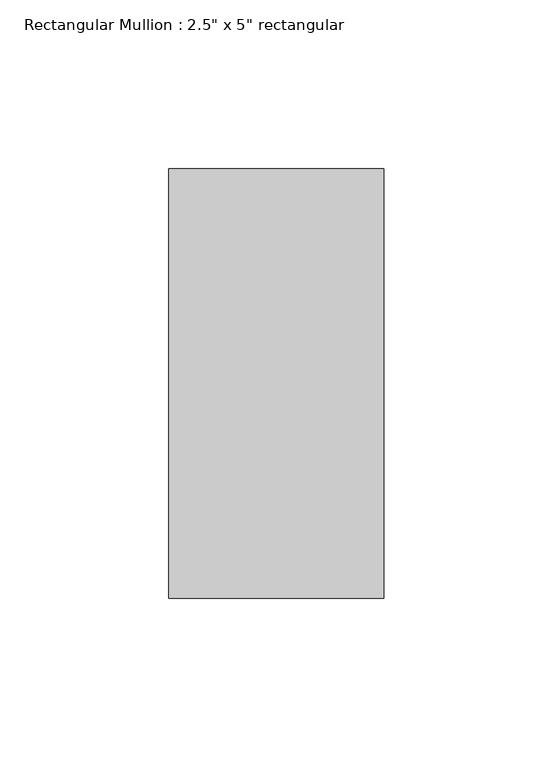
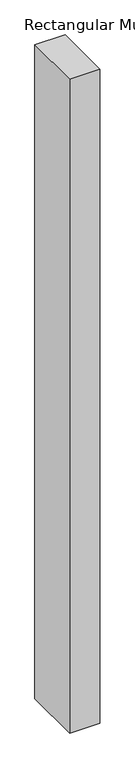
"""IFC4 building model written with IfcOpenShell, lengths in millimetres: member geometry."""

from ifc_helpers import new_model, si_unit, frame, origin, place, context, project, spatial, polyline, outline, extrude, source, transform, mapped, element, save


def member_9369ce3c(model_context):
    return source(origin(), model_context, "Body", "SweptSolid", [
        extrude(outline(polyline([(31.75, 63.5), (31.75, -63.5), (-31.75, -63.5), (-31.75, 63.5), (31.75, 63.5)])), frame((0.0, 0.0, -1455.9654832), z_axis=(0.0, 0.0, 1.0), x_axis=(1.0, 0.0, 0.0)), (0.0, 0.0, 1.0), 1455.9654832),
    ])


if __name__ == "__main__":
    model = new_model("IFC4")
    model_context = context("Model", 3, world=origin())
    ifc_project = project(units=[si_unit("LENGTHUNIT", "METRE", prefix="MILLI")], contexts=[model_context])
    site = spatial("IfcSite", under=ifc_project)
    building = spatial("IfcBuilding", under=site)
    placement = place(None, origin())
    member_shape = member_9369ce3c(model_context)
    element("IfcMember", 1, ObjectType="Rectangular Mullion : 2.5\" x 5\" rectangular", at=placement, inside=building, context=model_context, shape_type="MappedRepresentation", body=[
        mapped(member_shape, transform((0.0, 0.0, 0.0), x_axis=(1.0, 0.0, 0.0), y_axis=(0.0, 1.0, 0.0), z_axis=(0.0, 0.0, 1.0))),
    ])
    save(model, "model.ifc")

# Revit data of these elements
# Type "Rectangular Mullion : 2.5\" x 5\" rectangular"
#   built-in parameter 1007304 = 0.416667 (stored number, unit not read)
#   built-in parameter 1007301 = 0.104167 (stored number, unit not read)
#   built-in parameter 1007300 = 0.104167 (stored number, unit not read)
# Element 1 (IfcMember, "Rectangular Mullion : 2.5\" x 5\" rectangular")
#   Materials on its faces: "Aluminum"
# Materials
#   "Aluminum": class "Metal", colour RGB 247 247 247, transparency 0, Description = "Aluminum 6061", Cost = 0
